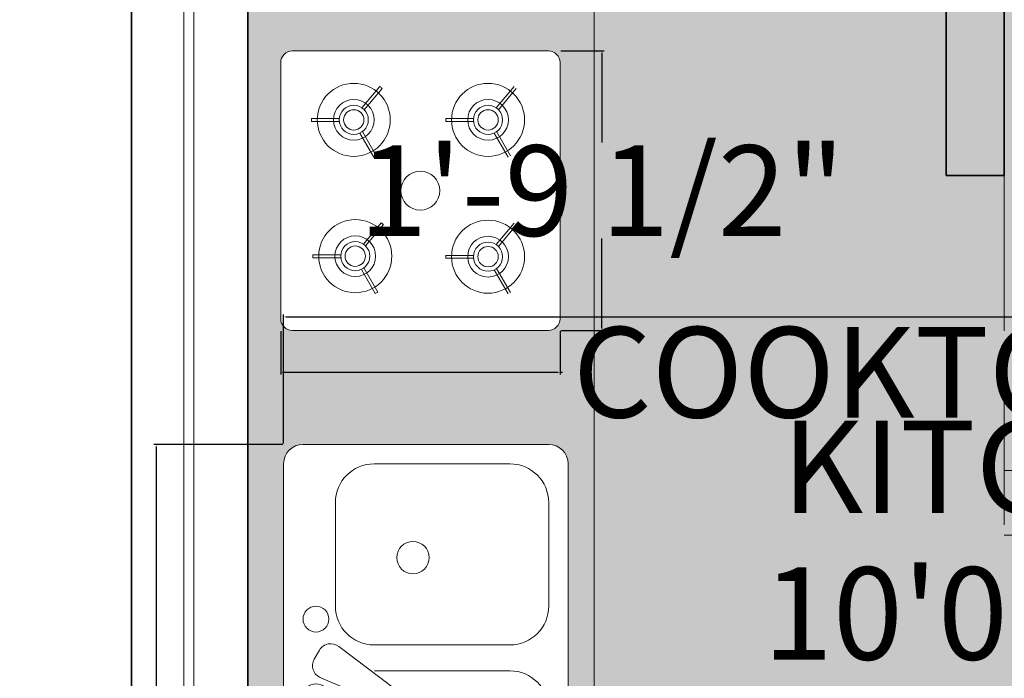
# Model space of a CAD drawing. Units: inches. Extents: x 1316 to 1777, y 813 to 1650.
# Tile 6 of 22: x 1368 to 1445, y 1284 to 1335. Entities that reach past the tile are written whole.
import ezdxf

# ---------------------------------------------------------------- set-up
doc = ezdxf.new("R2010")
doc.units = ezdxf.units.IN
doc.header["$MEASUREMENT"] = 0
doc.linetypes.add('ACAD_ISO02W100', pattern=[15, 12, -3])
for name, color, linetype, lineweight in [('A-ANNO-DIMS', 2, 'Continuous', 18), ('A-AREA-IDEN', 7, 'Continuous', 18), ('A-EQPM', 8, 'Continuous', 18), ('A-FLOR-CASE', 23, 'Continuous', 18), ('A-FLOR-CASE-PATT', 252, 'Continuous', 13), ('A-FLOR-FIXT', 8, 'Continuous', 18), ('A-WALL-OVHD', 250, 'ACAD_ISO02W100', 18), ('A-WALL-PATT', 250, 'Continuous', 13), ('furniture', 23, 'Continuous', 18), ('walls', 250, 'Continuous', 35), ('windows', 141, 'Continuous', 18)]:
    doc.layers.add(name, color=color, linetype=linetype, lineweight=lineweight)
doc.layers.add('A-FLOR-PATT', color=254, linetype='Continuous', lineweight=13, true_color=0xfeeab9)
doc.styles.add('ATT', font='TXT')
doc.styles.get("Standard").update_dxf_attribs({"font": 'arial.ttf'})
doc.dimstyles.get("Standard").update_dxf_attribs({"dimtxt": 7, "dimasz": 0.18, "dimexe": 0.18, "dimexo": 0.0625, "dimgap": 0.09, "dimtad": 0, "dimtih": 1, "dimtoh": 1, "dimzin": 0, "dimdsep": 46, "dimlunit": 3, "dimtxsty": 'Standard', "dimcen": 0.09, "dimadec": 0, "dimazin": 0, "dimtfac": 1, "dimtofl": 0, "dimtmove": 0, "dimatfit": 3, "dimfxl": 1, "dimtolj": 1, "dimtzin": 0, "dimarcsym": 0})

# ---------------------------------------------------------------- blocks, each defined once
blk = doc.blocks.new('15PSNK10')
at = {"color": 0, "linetype": 'ByBlock'}
for p, q in [((20.5, 16.5), (1.5, 16.5)), ((0, 15), (0, -15)), ((7, 15), (17.5, 15)), ((22, -15), (22, 15)), ((4, 4), (4, 12)), ((20.5, 12), (20.5, 4)), ((10.17820310567643, -3.566986483662404), (4.270020000000002, 0.8709410000000019)), ((17.5, 1), (7, 1)), ((2.365550999999996, -0.0988979999999984), (2.768423999999995, 0.5988979999999984)), ((7.038591832997624, -1), (17.5, -1)), ((2.880752999999998, -1.535340000000005), (9.678203105676431, -4.433012483662395)), ((9.678203105676431, -4.433012483662395), (10.17820310567643, -3.566986483662404)), ((4, -12), (4, -4)), ((20.5, -4), (20.5, -12)), ((17.5, -15), (7, -15)), ((1.5, -16.5), (20.5, -16.5))]:
    blk.add_line(p, q, dxfattribs=at)
for centre, radius in [((10, 7.75), 1.25), ((2.5, 3), 1), ((2.5, -3), 1), ((10, -7.75), 1.25)]:
    blk.add_circle(centre, radius, dxfattribs=at)
for centre, radius, start, end in [((1.5, 15), 1.5, 90, 180), ((20.5, 15), 1.5, 0, 90), ((7, 12), 3, 90, 180), ((17.5, 12), 3, 0, 90), ((7, 4), 3, 180, 270), ((17.5, 4), 3, 270, 0), ((3.634449000000003, 0.0988979999999984), 1, 50.537678, 150), ((3.231576000000004, -0.5988979999999984), 1, 150, 249.462322), ((17.5, -4), 3, 0, 90), ((7, -4), 3, 146.6070344853579, 180), ((7, -12), 3, 180, 270), ((17.5, -12), 3, 270, 0), ((1.5, -15), 1.5, 180, 270), ((20.5, -15), 1.5, 270, 0)]:
    blk.add_arc(centre, radius, start, end, dxfattribs=at)
at = {"color": 0, "linetype": 'ByBlock', "style": 'ATT'}
for tag, p, flags in [('ITEM', (0, -26), 3), ('ROOM_NUMBER', (0, -35), 1)]:
    blk.add_attdef(tag, p, '', height=6, dxfattribs=dict(at, flags=flags))
blk = doc.blocks.new('4bstove')
at = {"layer": 'furniture'}
for p, q in [((1452.734651100344, 1446.213675667939), (1452.734651100344, 1448.605619579717)), ((1452.984651100344, 1446.216662390849), (1452.984651100344, 1448.606641539671)), ((1464.44122432111, 1446.341246424268), (1464.44122432111, 1448.733190336046)), ((1464.69122432111, 1446.344233147178), (1464.69122432111, 1448.734212296)), ((1451.73906976938, 1444.448764170567), (1449.669037203066, 1443.253630311174)), ((1451.865811318356, 1444.233263303391), (1449.79463312554, 1443.037468016228)), ((1453.750175383867, 1444.079499707197), (1455.581487244284, 1442.54284660055)), ((1453.910173656299, 1444.271597038143), (1455.741945084313, 1442.734558308493)), ((1463.445642990145, 1444.576334926896), (1461.375610423832, 1443.381201067503)), ((1463.572384539122, 1444.36083405972), (1461.501206346306, 1443.165038772557)), ((1465.456748604633, 1444.207070463526), (1467.288060465049, 1442.670417356879)), ((1465.616746877065, 1444.399167794472), (1467.448518305079, 1442.862129064822)), ((1452.691937061862, 1434.805644860098), (1452.691937061862, 1437.197588771873)), ((1452.941937061862, 1434.808631583008), (1452.941937061862, 1437.19861073183)), ((1464.44122432111, 1434.805644860098), (1464.44122432111, 1437.197588771873)), ((1464.69122432111, 1434.808631583008), (1464.69122432111, 1437.19861073183)), ((1451.696355730898, 1433.040733362724), (1449.626323164584, 1431.845599503333)), ((1463.445642990145, 1433.040733362724), (1461.375610423832, 1431.845599503333)), ((1451.823097279874, 1432.82523249555), (1449.751919087058, 1431.629437208387)), ((1453.707461345386, 1432.671468899352), (1455.538773205802, 1431.134815792708)), ((1453.867459617818, 1432.863566230298), (1455.699231045831, 1431.326527500652)), ((1463.572384539122, 1432.82523249555), (1461.501206346306, 1431.629437208387)), ((1465.456748604633, 1432.671468899352), (1467.288060465049, 1431.134815792708)), ((1465.616746877065, 1432.863566230298), (1467.448518305079, 1431.326527500652))]:
    blk.add_line(p, q, dxfattribs=at)
for points in [[(1447.502363082413, 1427.379846129004), (1469.502363082413, 1427.379846129004, 0.4142135623730951), (1470.502363082413, 1428.379846129004), (1470.502363082413, 1450.379846129006, 0.4142135623730951), (1469.502363082413, 1451.379846129006), (1447.502363082413, 1451.379846129006, 0.4142135623730966), (1446.502363082413, 1450.379846129006), (1446.502363082413, 1428.379846129004, 0.4142135623730935)], [(1453.749508788236, 1444.971524377983, 1), (1451.999508788236, 1444.971524377983, 1)], [(1465.456082009002, 1445.099095134312, 1), (1463.706082009001, 1445.099095134312, 1)], [(1453.706794749754, 1433.563493570142, 1), (1451.956794749754, 1433.563493570142, 1)], [(1465.456082009002, 1433.563493570142, 1), (1463.706082009001, 1433.563493570142, 1)]]:
    blk.add_lwpolyline(points, format="xyb", close=True, dxfattribs=at)
for points in [[(1454.124508788236, 1444.971524377983, 0.9999999673531919), (1451.624508788236, 1444.971524377983, 0.9999999673531919), (1454.124508788236, 1444.971524377983, 0.9999999673531919)], [(1465.831082009002, 1445.099095134312, 1), (1463.331082009001, 1445.099095134312, 1), (1465.831082009002, 1445.099095134312, 1)], [(1454.081794749754, 1433.563493570142, 0.9999999673531919), (1451.581794749754, 1433.563493570142, 0.9999999673531919), (1454.081794749754, 1433.563493570142, 0.9999999673531919)], [(1465.831082009002, 1433.563493570142, 1), (1463.331082009001, 1433.563493570142, 1), (1465.831082009002, 1433.563493570142, 1)]]:
    blk.add_lwpolyline(points, format="xyb", dxfattribs=at)
for centre, radius in [((1452.874508788236, 1444.971524377983), 3.136785408586831), ((1464.581082009001, 1445.099095134312), 3.136785408586831), ((1452.874508788236, 1444.971524377983), 1.75), ((1464.581082009001, 1445.099095134312), 1.75), ((1458.502363082413, 1439.379846129004), 1.670451188942094), ((1452.831794749754, 1433.563493570142), 3.136785408586831), ((1464.581082009001, 1433.563493570142), 3.136785408586831), ((1452.831794749754, 1433.563493570142), 1.75), ((1464.581082009001, 1433.563493570142), 1.75)]:
    blk.add_circle(centre, radius, dxfattribs=at)
for centre, start, end in [((1452.874508788236, 1444.971524377983), 88.2644962424337, 92.20393308675509), ((1464.581082009001, 1445.099095134312), 88.2644962424337, 92.20393308675509), ((1452.874508788236, 1444.971524377983), 208.1879938332412, 212.1274126783975), ((1464.581082009001, 1445.099095134312), 208.1879938332412, 212.1274126783975), ((1452.874508788236, 1444.971524377983), 318.1018185131579, 322.0412255005968), ((1464.581082009001, 1445.099095134312), 318.1018185131579, 322.0412255005968), ((1452.831794749754, 1433.563493570142), 88.2644962424337, 92.20393308675509), ((1464.581082009001, 1433.563493570142), 88.2644962424337, 92.20393308675509)]:
    blk.add_arc(centre, 3.636785408586831, start, end, dxfattribs=at)
blk = doc.blocks.new('stove')
at = {"layer": 'furniture', "xscale": 0.9, "yscale": 0.9, "zscale": 0.9, "rotation": 89.99999999999999}
blk.add_blockref('4bstove', (1295.441862106323, -1312.652126789093), dxfattribs=at)
blk = doc.blocks.new('*D36')
at = {"layer": 'A-ANNO-DIMS', "color": 0, "lineweight": -2, "transparency": 16777216}
for p, q in [((1416.108011424953, 1349.392697936214), (1416.108011424953, 1345.951925450247)), ((1438.2631613314, 1349.392697936214), (1438.2631613314, 1345.951925450247)), ((1416.288011424953, 1346.131925450247), (1438.0831613314, 1346.131925450247)), ((1438.2631613314, 1346.131925450247), (1438.443161331401, 1346.131925450247))]:
    blk.add_line(p, q, dxfattribs=at)
at = {"layer": 'A-ANNO-DIMS', "color": 0, "transparency": 16777216}
for points in [[(1416.288011424953, 1346.161925450247), (1416.288011424953, 1346.101925450247), (1416.108011424953, 1346.131925450247)], [(1438.0831613314, 1346.161925450247), (1438.0831613314, 1346.101925450247), (1438.2631613314, 1346.131925450247)]]:
    blk.add_solid(points, dxfattribs=at)
at = {"layer": 'Defpoints', "color": 0, "transparency": 16777216}
for p in [(1416.108011424953, 1349.455197936214), (1438.2631613314, 1349.455197936214), (1438.2631613314, 1346.131925450247)]:
    blk.add_point(p, dxfattribs=at)
at = {"layer": 'A-ANNO-DIMS', "color": 0, "transparency": 16777216, "insert": (1493.434934864825, 1346.131925450247), "char_height": 7, "attachment_point": 5}
blk.add_mtext('\\A1;WALL BASIN 1\'-10" TYP.', dxfattribs=at)
blk = doc.blocks.new('*D40')
at = {"layer": 'A-ANNO-DIMS', "color": 0, "lineweight": -2, "transparency": 16777216}
for p, q in [((1388.838253781963, 1302.162642632137), (1388.838253781963, 1312.140959778822)), ((1389.018253781963, 1311.960959778821), (1454.39703475986, 1311.960959778821)), ((1454.57703475986, 1302.162642632137), (1454.57703475986, 1312.140959778822)), ((1454.57703475986, 1311.960959778821), (1454.757034759859, 1311.960959778821))]:
    blk.add_line(p, q, dxfattribs=at)
at = {"layer": 'A-ANNO-DIMS', "color": 0, "transparency": 16777216}
for points in [[(1389.018253781963, 1311.990959778821), (1389.018253781963, 1311.930959778822), (1388.838253781963, 1311.960959778821)], [(1454.39703475986, 1311.990959778821), (1454.39703475986, 1311.930959778822), (1454.57703475986, 1311.960959778821)]]:
    blk.add_solid(points, dxfattribs=at)
at = {"layer": 'Defpoints', "color": 0, "transparency": 16777216}
for p in [(1454.57703475986, 1311.960959778821), (1388.838253781963, 1302.100142632137), (1454.57703475986, 1302.100142632137)]:
    blk.add_point(p, dxfattribs=at)
at = {"layer": 'A-ANNO-DIMS', "color": 0, "transparency": 16777216, "insert": (1507.740963818523, 1311.960959778821), "char_height": 7, "attachment_point": 5}
blk.add_mtext('\\A1;KITCHEN SINK 5\'-5 1/2"', dxfattribs=at)
blk = doc.blocks.new('*D41')
at = {"layer": 'A-ANNO-DIMS', "color": 0, "lineweight": -2, "transparency": 16777216}
for p, q in [((1388.775753781963, 1302.100142632137), (1378.797436635279, 1302.100142632137)), ((1378.977436635279, 1301.920142632137), (1378.977436635279, 1279.143834211486)), ((1378.977436635279, 1249.068153348815), (1378.977436635279, 1271.844461769467)), ((1388.775753781963, 1248.888153348815), (1378.797436635279, 1248.888153348815))]:
    blk.add_line(p, q, dxfattribs=at)
at = {"layer": 'A-ANNO-DIMS', "color": 0, "transparency": 16777216}
for points in [[(1378.947436635279, 1301.920142632137), (1379.007436635279, 1301.920142632137), (1378.977436635279, 1302.100142632137)], [(1378.947436635279, 1249.068153348815), (1379.007436635279, 1249.068153348815), (1378.977436635279, 1248.888153348815)]]:
    blk.add_solid(points, dxfattribs=at)
at = {"layer": 'Defpoints', "color": 0, "transparency": 16777216}
for p in [(1378.977436635279, 1302.100142632137), (1388.838253781963, 1302.100142632137), (1388.838253781963, 1248.888153348815)]:
    blk.add_point(p, dxfattribs=at)
at = {"layer": 'A-ANNO-DIMS', "color": 0, "transparency": 16777216, "insert": (1378.977436635279, 1275.494147990476), "char_height": 7, "attachment_point": 5}
blk.add_mtext('\\A1;4\'-5"', dxfattribs=at)
blk = doc.blocks.new('*D42')
at = {"layer": 'A-ANNO-DIMS', "color": 0, "lineweight": -2, "transparency": 16777216}
for p, q in [((1388.610422891291, 1310.852265372921), (1388.610422891291, 1307.49476537292)), ((1410.210422891293, 1310.852265372921), (1410.210422891293, 1307.49476537292)), ((1388.790422891291, 1307.674765372921), (1410.030422891293, 1307.674765372921)), ((1410.210422891293, 1307.674765372921), (1410.390422891293, 1307.674765372921))]:
    blk.add_line(p, q, dxfattribs=at)
at = {"layer": 'A-ANNO-DIMS', "color": 0, "transparency": 16777216}
for points in [[(1388.790422891291, 1307.704765372921), (1388.790422891291, 1307.644765372921), (1388.610422891291, 1307.674765372921)], [(1410.030422891293, 1307.704765372921), (1410.030422891293, 1307.644765372921), (1410.210422891293, 1307.674765372921)]]:
    blk.add_solid(points, dxfattribs=at)
at = {"layer": 'Defpoints', "color": 0, "transparency": 16777216}
for p in [(1388.610422891291, 1310.914765372921), (1410.210422891293, 1310.914765372921), (1410.210422891293, 1307.674765372921)]:
    blk.add_point(p, dxfattribs=at)
at = {"layer": 'A-ANNO-DIMS', "color": 0, "transparency": 16777216, "insert": (1453.707571595249, 1307.674765372921), "char_height": 7, "attachment_point": 5}
blk.add_mtext('\\A1;COOKTOP 1\'-9 1/2"', dxfattribs=at)
blk = doc.blocks.new('*D43')
at = {"layer": 'A-ANNO-DIMS', "color": 0, "lineweight": -2, "transparency": 16777216}
for p, q in [((1410.272922891293, 1332.514765372921), (1413.630422891294, 1332.514765372921)), ((1413.450422891294, 1332.334765372921), (1413.450422891294, 1325.42413781494)), ((1413.450422891294, 1311.094765372921), (1413.450422891294, 1318.005392930902)), ((1410.272922891293, 1310.914765372921), (1413.630422891294, 1310.914765372921))]:
    blk.add_line(p, q, dxfattribs=at)
at = {"layer": 'A-ANNO-DIMS', "color": 0, "transparency": 16777216}
for points in [[(1413.420422891294, 1332.334765372921), (1413.480422891294, 1332.334765372921), (1413.450422891294, 1332.514765372921)], [(1413.420422891294, 1311.094765372921), (1413.480422891294, 1311.094765372921), (1413.450422891294, 1310.914765372921)]]:
    blk.add_solid(points, dxfattribs=at)
at = {"layer": 'Defpoints', "color": 0, "transparency": 16777216}
for p in [(1410.210422891293, 1332.514765372921), (1413.450422891294, 1332.514765372921), (1410.210422891293, 1310.914765372921)]:
    blk.add_point(p, dxfattribs=at)
at = {"layer": 'A-ANNO-DIMS', "color": 0, "transparency": 16777216, "insert": (1413.450422891294, 1321.714765372921), "char_height": 7, "attachment_point": 5}
blk.add_mtext('\\A1;1\'-9 1/2"', dxfattribs=at)

msp = doc.modelspace()

# ---------------------------------------------------------------- hatches: boundary and pattern name
at = {"layer": 'A-FLOR-CASE-PATT'}
h = msp.add_hatch(color=256, dxfattribs=at)
h.dxf.hatch_style = 1
h.paths.add_polyline_path([(1412.858226839809, 1346.928610372446), (1440.064450217018, 1346.928610372446), (1440.064450217018, 1365.369300926962), (1438.2631613314, 1365.369300926962), (1438.2631613314, 1349.455197936214), (1416.108011424953, 1349.455197936214), (1416.108011424953, 1365.369300926962), (1386.064450217018, 1365.369300926962), (1386.064450217018, 1245.369300926962), (1412.858226839809, 1245.369300926962)])
h.paths.add_polyline_path([(1409.310422891292, 1332.514765372921, -0.4142135623730951), (1410.210422891292, 1331.614765372921), (1410.210422891292, 1311.814765372921, -0.414213562373094), (1409.310422891292, 1310.914765372921), (1389.51042289129, 1310.914765372921, -0.4142135623730959), (1388.61042289129, 1311.814765372921), (1388.61042289129, 1331.614765372921, -0.4142135623730951), (1389.51042289129, 1332.514765372921)], flags=16)
h.paths.add_polyline_path([(1395.986900854525, 1329.42133126595), (1396.276368249055, 1329.76630507332, -0.0171905986958355), (1396.448908786205, 1329.621893017294), (1396.159470211814, 1329.276953556429, -0.2116405901053515), (1397.086205654243, 1327.18561240685, -0.2564460938474173), (1395.778569555149, 1324.8037474367), (1396.003749512095, 1324.413724310425, -0.0171906504505625), (1395.809203446643, 1324.300687980197), (1395.584072921188, 1324.69062548862, -0.550570801787435), (1391.442799396982, 1327.059740487748), (1390.992413104956, 1327.059740487748, -0.0171907290098312), (1390.991493340996, 1327.284740487748), (1391.441732803486, 1327.284740487748, -0.6105283005508269)], flags=0)
h.paths.add_polyline_path([(1395.838098786515, 1327.18561240685, -1), (1392.688098786514, 1327.18561240685, -1)], flags=0)
h.paths.add_polyline_path([(1394.263098786514, 1328.310612406851, -1), (1394.263098786514, 1326.06061240685, -1)], flags=0)
h.paths.add_polyline_path([(1394.263098786514, 1327.973112406851, -1), (1394.263098786514, 1326.39811240685, -1)], flags=0)
h.paths.add_polyline_path([(1407.468247061996, 1327.18561240685, -0.9779444631718501), (1401.824840804736, 1327.059740487748), (1401.37445451271, 1327.059740487748, -0.0171907290098312), (1401.373534748749, 1327.284740487748), (1401.823774211239, 1327.284740487748, -0.9825922263687022)], flags=0)
h.paths.add_polyline_path([(1406.220140194268, 1327.18561240685, -1), (1403.070140194268, 1327.18561240685, -1)], flags=0)
h.paths.add_polyline_path([(1404.645140194268, 1328.310612406851, -1), (1404.645140194268, 1326.06061240685, -1)], flags=0)
h.paths.add_polyline_path([(1404.645140194268, 1327.973112406851, -1), (1404.645140194268, 1326.39811240685, -1)], flags=0)
h.paths.add_polyline_path([(1400.91382896134, 1321.714765372921, -1), (1397.907016821244, 1321.714765372921, -1)], flags=0)
h.paths.add_polyline_path([(1396.101714535222, 1318.885415367262), (1396.391181929752, 1319.230389174631, -0.0171905986957908), (1396.563722466901, 1319.085977118605), (1396.274283892511, 1318.74103765774, -0.2116405901053402), (1397.201019334939, 1316.649696508162, -0.2564460938474829), (1395.893383235845, 1314.267831538011), (1396.11856319279, 1313.877808411735, -0.0171906504505387), (1395.924017127339, 1313.764772081509), (1395.698886601884, 1314.154709589932, -0.5505708017872751), (1391.557613077679, 1316.523824589059), (1391.107226785653, 1316.523824589059, -0.0171907290098486), (1391.106307021692, 1316.748824589059), (1391.556546484182, 1316.748824589059, -0.6105283005510082)], flags=0)
h.paths.add_polyline_path([(1395.952912467211, 1316.649696508162, -1), (1392.802912467211, 1316.649696508162, -1)], flags=0)
h.paths.add_polyline_path([(1407.468247061996, 1316.611253873528, -0.9779444631716472), (1401.824840804736, 1316.485381954425), (1401.37445451271, 1316.485381954425, -0.0171907290098486), (1401.373534748749, 1316.710381954425), (1401.823774211239, 1316.710381954425, -0.9825922263688615)], flags=0)
h.paths.add_polyline_path([(1394.377912467211, 1317.774696508162, -0.9999999703822144), (1394.377912467211, 1315.524696508162, -0.9999999703822144)], flags=0)
h.paths.add_polyline_path([(1394.377912467211, 1317.437196508162, -1), (1394.377912467211, 1315.862196508162, -1)], flags=0)
h.paths.add_polyline_path([(1406.220140194268, 1316.611253873528, -1), (1403.070140194268, 1316.611253873528, -1)], flags=0)
h.paths.add_polyline_path([(1404.645140194268, 1315.486253873528, -0.9999999703822144), (1404.645140194268, 1317.736253873528, -0.9999999703822144)], flags=0)
h.paths.add_polyline_path([(1404.645140194268, 1317.398753873528, -1), (1404.645140194268, 1315.823753873528, -1)], flags=0)
h.paths.add_polyline_path([(1409.338253781963, 1302.100142632137, -0.4142135623730951), (1410.838253781963, 1300.600142632137), (1410.838253781963, 1270.600142632137, -0.4142135623730951), (1409.338253781963, 1269.100142632137), (1390.338253781963, 1269.100142632137, -0.4142135623730951), (1388.838253781963, 1270.600142632137), (1388.838253781963, 1300.600142632137, -0.4142135623730951), (1390.338253781963, 1302.100142632137)], flags=16)
h.paths.add_polyline_path([(1395.838253781963, 1300.600142632137), (1406.338253781963, 1300.600142632137, -0.4142135623730951), (1409.338253781963, 1297.600142632137), (1409.338253781963, 1289.600142632137, -0.4142135623730951), (1406.338253781963, 1286.600142632137), (1395.838253781963, 1286.600142632137, -0.4142135623730951), (1392.838253781963, 1289.600142632137), (1392.838253781963, 1297.600142632137, -0.4142135623730951)], flags=0)
h.paths.add_polyline_path([(1400.088253781963, 1293.350142632137, -1), (1397.588253781963, 1293.350142632137, -1)], flags=0)
h.paths.add_polyline_path([(1392.338253781963, 1288.600142632137, -1), (1390.338253781963, 1288.600142632137, -1)], flags=0)
h.paths.add_polyline_path([(1393.037126479862, 1286.524525876857), (1399.01645688764, 1282.033156148475), (1398.51645688764, 1281.167130148475), (1391.719002681245, 1284.064804380225, -0.4631994748411593), (1391.203386694108, 1285.500520483254), (1391.606259694108, 1286.198316483253, -0.4369421512224802)], flags=0)
h.paths.add_polyline_path([(1392.338253781963, 1282.600142632137, -1), (1390.338253781963, 1282.600142632137, -1)], flags=0)
h.paths.add_polyline_path([(1400.088253781963, 1277.850142632137, -1), (1397.588253781963, 1277.850142632137, -1)], flags=0)
at = {"layer": 'A-FLOR-PATT'}
h = msp.add_hatch(color=256, dxfattribs=at)
h.dxf.hatch_style = 1
h.paths.add_polyline_path([(1567.673142217696, 1281.369300926962), (1651.673142217696, 1281.369300926962), (1651.673142217696, 1365.369300926962), (1597.673142217696, 1365.369300926962), (1597.673142217696, 1429.869300926962), (1570.345136951899, 1429.869300926962), (1570.345136951899, 1471.869300926962), (1510.345136951899, 1471.869300926962), (1510.345136951899, 1429.869300926962), (1444.564450217018, 1429.869300926962), (1444.564450217018, 1322.882360660317), (1444.564450217018, 1300.087519887597), (1510.564450217018, 1300.087519887597), (1510.564450217018, 1295.093869264817), (1510.564450217018, 1240.869300926962), (1386.064450217018, 1240.869300926962), (1386.064450217018, 1171.184826128129), (1400.961298831769, 1171.184826128129), (1400.961298831769, 1106.74181853581), (1386.064450217018, 1106.74181853581), (1386.064450217018, 1072.869300926962), (1510.564450217018, 1072.869300926962), (1510.564450217018, 1040.172951843256), (1541.068383692007, 1040.172951843256, -0.367085007058701), (1572.764174999282, 1069.546549507821), (1572.764174999282, 1069.578525976929), (1574.225256623933, 1069.578525976929), (1574.225256623933, 1040.172951843256), (1616.037285953149, 1040.172951843256), (1616.037285953149, 1086.627161740109), (1616.037285953149, 1103.704513499145), (1613.066060418845, 1105.234780569291), (1616.037285953149, 1106.685539866415), (1616.037285953149, 1123.869300926962), (1567.673142217696, 1123.869300926962)])
h.paths.add_polyline_path([(1508.987494855724, 1198.018101264616), (1511.117481528599, 1198.018101264616), (1511.117481528599, 1200.148087937491), (1532.594847146751, 1200.148087937491), (1532.594847146751, 1198.018101264616), (1534.724833819626, 1198.018101264616), (1534.724833819626, 1176.008238978245), (1530.464860473877, 1176.008238978245), (1530.464860473877, 1176.71823453587), (1513.247468201473, 1176.71823453587), (1513.247468201473, 1176.008238978245), (1508.987494855724, 1176.008238978245)], flags=16)
h.paths.add_polyline_path([(1505.978911344017, 1151.314990471522), (1521.503967005494, 1151.314990471522), (1521.503967005494, 1123.622553675171), (1505.978911344017, 1123.622553675171)], flags=16)
h.paths.add_polyline_path([(1507.734238645614, 1150.100746953806, -1), (1506.932299902515, 1150.100746953806, -1)], flags=0)
h.paths.add_polyline_path([(1512.288074001727, 1138.353334368216), (1512.279600715468, 1138.392440283947), (1512.219350358134, 1138.376242249414)], flags=0)
h.paths.add_polyline_path([(1511.538708600003, 1138.926307509397), (1511.801586230713, 1138.967144364025), (1511.816822451641, 1139.269704188439), (1511.606794574277, 1139.246286533845)], flags=0)
h.paths.add_polyline_path([(1513.744555260512, 1140.234298321423), (1513.680232363733, 1139.885116881769), (1514.013725426534, 1140.045442118172), (1513.85452204526, 1140.307851476896)], flags=0)
h.paths.add_polyline_path([(1513.759454991183, 1139.088508933479), (1514.004707571892, 1139.255238426424), (1513.806733823314, 1139.482778214552), (1513.564128907831, 1139.327271464974)], flags=0)
h.paths.add_polyline_path([(1514.219475210051, 1138.385213274156), (1514.335730050378, 1138.330012877603), (1514.544443105969, 1138.319719602207), (1514.802071501717, 1138.873746829037), (1514.451386945615, 1138.715560522777)], flags=0)
h.paths.add_polyline_path([(1514.576784523415, 1137.439218133731), (1514.572807725035, 1137.400121795131), (1514.699202201671, 1137.400121795131), (1514.696265725507, 1137.401958254237)], flags=0)
h.paths.add_polyline_path([(1512.259630054145, 1136.199252443718), (1512.198645006043, 1136.399020086717), (1512.031969302785, 1136.324884611944), (1512.095408670439, 1136.101205019573), (1512.257489338984, 1136.192116726515)], flags=0)
h.paths.add_polyline_path([(1512.643663084783, 1137.273739653883), (1512.355504649132, 1137.230281342332), (1512.431954114942, 1137.048783229095), (1512.702875297586, 1137.092989450977)], flags=0)
h.paths.add_polyline_path([(1513.048588650928, 1137.592520798729), (1512.979298324136, 1137.799799709794), (1512.842806872769, 1137.757466697763), (1512.887278702865, 1137.556025839099)], flags=0)
h.paths.add_polyline_path([(1513.269281623239, 1138.555876366321), (1513.570749546786, 1137.962332598873), (1513.458764523686, 1136.814048268166), (1513.212081965274, 1137.877990637943), (1513.032322366809, 1138.442602014432)], flags=0)
h.paths.add_polyline_path([(1514.891020715756, 1136.377090047208), (1514.695899864911, 1136.400535518201), (1514.682939550409, 1136.245500587688), (1514.870369662043, 1136.165423867704)], flags=0)
h.paths.add_polyline_path([(1514.142311807212, 1137.292647657223), (1514.047049214511, 1136.74320071616), (1514.270411313405, 1136.750949401328), (1514.327746372416, 1137.265481105849)], flags=0)
h.paths.add_polyline_path([(1515.361925908058, 1138.975942407129), (1515.333738674027, 1138.638448296537), (1515.595602136156, 1138.588081597507), (1515.627104749056, 1138.931608018565)], flags=0)
h.paths.add_polyline_path([(1537.284795120854, 1177.912388692567), (1537.994790678479, 1177.912388692567), (1537.994790678479, 1195.129780964971), (1537.284795120854, 1195.129780964971), (1537.284795120854, 1199.38975431072), (1559.294657407225, 1199.38975431072), (1559.294657407225, 1197.259767637845), (1561.4246440801, 1197.259767637845), (1561.4246440801, 1175.782402019693), (1559.294657407225, 1175.782402019693), (1559.294657407225, 1173.652415346818), (1559.378615070445, 1173.652415346818), (1559.378615070445, 1171.514303738793), (1561.51672667847, 1171.514303738793), (1561.51672667847, 1098.818509065945), (1559.378615070445, 1098.818509065945), (1559.378615070445, 1096.68039745792), (1537.284795120854, 1096.68039745792), (1537.284795120854, 1100.95662067397), (1537.997498990196, 1100.95662067397), (1537.997498990196, 1169.376192130768), (1537.284795120854, 1169.376192130768), (1537.284795120854, 1173.652415346818)], flags=16)
h.paths.add_polyline_path([(1518.623279367581, 1345.565265318288), (1519.133216999197, 1345.479657117201), (1519.133247129367, 1345.484585273925), (1518.623292796693, 1345.567461813277)], flags=16)
h.paths.add_polyline_path([(1518.798043157878, 1374.150014517315), (1519.307980789494, 1374.064406316228), (1519.308010919664, 1374.069334472953), (1518.79805658699, 1374.152211012305)], flags=16)
h.paths.add_polyline_path([(1537.763945546351, 1413.501272593833), (1537.678419015976, 1412.991334462891), (1537.683273643974, 1412.991304782267), (1537.76615767817, 1413.501259069119)], flags=16)
h.paths.add_polyline_path([(1572.904903294898, 1373.821409718101), (1573.926762419731, 1373.974678074354), (1574.026627442758, 1390.308820473798), (1573.007147246318, 1390.474521481455), (1573.006718884663, 1390.474591095266)], flags=16)
h.paths.add_polyline_path([(1572.730139504601, 1345.236660519073), (1573.751998629434, 1345.389928875326), (1573.851863652461, 1361.72407127477), (1572.832383456021, 1361.889772282427), (1572.831955094366, 1361.889841896238)], flags=16)
h.paths.add_polyline_path([(1537.210658487583, 1322.64259197221), (1537.363943428096, 1321.620732745983), (1553.69808582754, 1321.520867722956), (1553.863838585734, 1322.540776390265)], flags=16)
h.paths.add_polyline_path([(1535.907853535946, 1331.328394679552), (1527.214399285865, 1331.381545435045), (1527.663791889487, 1404.885186232545), (1564.415612288236, 1404.660489930734), (1563.966219684615, 1331.156849133235), (1555.272745017813, 1331.210000013553), (1553.946716560728, 1323.050730714162), (1537.134020158137, 1323.153521560007)], flags=16)
h.paths.add_polyline_path([(1536.149948378398, 1336.502989385165), (1536.235164066325, 1337.571577967879), (1536.323287084786, 1338.628101895201), (1536.410786509507, 1339.662781903015), (1536.494625364907, 1340.6698173033), (1536.573878305868, 1341.65983134291), (1536.648126641431, 1342.647834135966), (1536.716972722469, 1343.648937760143), (1536.780017027388, 1344.677948027938), (1536.836830656389, 1345.749875115879), (1536.91349345135, 1347.47536960008), (1536.930181129876, 1348.082213381731), (1536.86671979596, 1346.313806322279), (1536.754065794645, 1344.188314997416), (1536.618602559507, 1342.21851898877), (1536.494625364906, 1340.669817303289), (1536.410786509508, 1339.662781903024), (1536.323287084785, 1338.628101895196), (1536.235164066325, 1337.571577967878), (1536.149948378398, 1336.502989385167), (1536.071202820108, 1335.432319400725), (1536.002480605875, 1334.369653419014), (1535.917201218224, 1332.754159960459), (1535.909282823342, 1332.307756473361), (1535.96435308899, 1333.780079645636), (1536.071202820108, 1335.432319400726)], flags=0)
h.paths.add_polyline_path([(1540.411728678358, 1338.345220732376), (1540.538507986221, 1339.036732867615), (1540.667450686668, 1339.758144792479), (1540.798139602249, 1340.51803480286), (1540.930104638842, 1341.324675241543), (1541.06290820131, 1342.186644529235), (1541.195663950278, 1343.109256879628), (1541.325751198274, 1344.084667215432), (1541.450112594895, 1345.102072455087), (1541.565699126105, 1346.150363189455), (1541.669432399664, 1347.218634373414), (1541.758274858692, 1348.295980712192), (1541.829158319786, 1349.371497098253), (1541.87902418423, 1350.434176273261), (1541.905658245644, 1351.475864398132), (1541.910264078201, 1352.499718972741), (1541.894848813054, 1353.511751165878), (1541.861450207875, 1354.517971959091), (1541.812104772023, 1355.524188157142), (1541.748831093802, 1356.536615043187), (1541.673675267255, 1357.560957271187), (1541.551221046702, 1359.062282646612), (1541.495486505545, 1359.670454934914), (1541.588655256529, 1358.603328035907), (1541.721318618915, 1356.976835527602), (1541.846114060333, 1354.980013725856), (1541.912433480836, 1352.981966815021), (1541.903299375855, 1350.951498912638), (1541.805645357175, 1348.870418133965), (1541.627733180341, 1346.712969607265), (1541.39605931794, 1344.611846225434), (1541.135168242209, 1342.655652549989), (1540.871929016276, 1340.947082961546), (1540.617179283622, 1339.465841984599), (1540.411728678363, 1338.345220732389), (1540.287580984743, 1337.67502977883), (1540.166494164132, 1337.01788791383), (1540.048925605183, 1336.365114503449), (1539.936674201221, 1335.710368832696), (1539.836864251217, 1335.055036635329), (1539.758020939376, 1334.402536924379), (1539.708629238703, 1333.756391050932), (1539.697173498044, 1333.120018277682), (1539.75093556766, 1332.162191347439), (1539.822087714565, 1331.89006440645), (1539.690956844971, 1332.774679737417), (1539.713650637448, 1334.035332547662), (1539.86680860596, 1335.30285325234), (1540.085210789094, 1336.576760560778), (1540.287580984743, 1337.67502977883)], flags=0)
h.paths.add_polyline_path([(1545.598581542273, 1331.583674047033), (1545.601408931398, 1331.616855477121), (1545.614142276281, 1331.689058908809), (1545.736718477884, 1332.197227143153), (1545.766951209007, 1332.331509735297), (1545.840044120643, 1332.681341212682), (1545.924609388668, 1333.114205605127), (1546.015565858785, 1333.613901317454), (1546.107830504227, 1334.163920489319), (1546.196310713542, 1334.747857411176), (1546.27592408412, 1335.349306311069), (1546.341588213349, 1335.951861417042), (1546.388220074462, 1336.539014868746), (1546.411904372759, 1337.098233262493), (1546.413511757999, 1337.631655211558), (1546.395048737181, 1338.145189796344), (1546.358553067975, 1338.644847998394), (1546.30606313221, 1339.136742887642), (1546.239595021565, 1339.626681393686), (1546.161196702551, 1340.120674435653), (1546.072884891005, 1340.624631031533), (1545.887738197254, 1341.63015699768), (1545.717659533451, 1342.62070013092), (1545.546853733249, 1343.94500888803), (1545.431881256549, 1345.533720124316), (1545.403899849759, 1347.401905451854), (1545.417510423816, 1348.013069267128), (1545.410556413592, 1346.957478372932), (1545.425070640934, 1345.988432507364), (1545.462877367243, 1345.105410056077), (1545.521092971858, 1344.300975918152), (1545.595702123642, 1343.566272620922), (1545.68263719895, 1342.892238827028), (1545.777872657803, 1342.270017126221), (1545.877351709551, 1341.690648207114), (1545.977037981224, 1341.145172633476), (1546.133225269608, 1340.296924301995), (1546.32712189736, 1339.07516870602), (1546.43378476773, 1337.614859053002), (1546.377188266119, 1336.278538916938), (1546.246417261819, 1335.078542247844), (1546.032296532176, 1333.665423983985), (1545.840044120643, 1332.681341212682), (1545.766951209007, 1332.331509735297)], flags=0)
h.paths.add_polyline_path([(1551.802739251137, 1337.655775652498), (1551.96257269545, 1338.249893918501), (1552.102195298518, 1338.801154932478), (1552.224958021371, 1339.338328209144), (1552.330696453755, 1339.864579612065), (1552.418402861907, 1340.377056720641), (1552.487067639598, 1340.872600849098), (1552.535672844225, 1341.34835963925), (1552.563199284875, 1341.801276556129), (1552.568639227787, 1342.228499179132), (1552.550972857889, 1342.626868884903), (1552.509678498417, 1342.994551203202), (1552.446288501197, 1343.33337442512), (1552.362792521005, 1343.646491244529), (1552.261208966661, 1343.936747902882), (1552.143557495304, 1344.207194818415), (1552.011836098078, 1344.460678357413), (1551.868075265113, 1344.700350964085), (1551.746105860759, 1344.881722683215), (1550.887297650741, 1346.05192221882), (1550.42788872704, 1347.125680184261), (1550.183287427721, 1348.353333686171), (1550.047936052465, 1349.632359022536), (1549.978096005541, 1351.223542107026), (1549.974102148838, 1353.140827975589), (1549.989226669163, 1353.748427546368), (1549.975058438592, 1352.681752708607), (1549.977087298692, 1351.70778065901), (1549.995607655661, 1350.824569845699), (1550.030618304039, 1350.026913573531), (1550.082058657804, 1349.309911787039), (1550.149928759809, 1348.668561967865), (1550.234168024029, 1348.097964060535), (1550.334775869163, 1347.593013458303), (1550.451691709185, 1347.148810105696), (1550.584412233058, 1346.759844100773), (1550.73038050297, 1346.418678345312), (1550.88655602074, 1346.117266144286), (1551.049909745336, 1345.847764917032), (1551.217401178577, 1345.602127968521), (1551.385990446439, 1345.372410692116), (1551.55262809021, 1345.150770631988), (1552.000038284146, 1344.537104232464), (1552.453505275841, 1343.494713960715), (1552.591463897673, 1342.266339273388), (1552.508711326437, 1340.904737898757), (1552.245597777252, 1339.367339734202), (1551.924893638995, 1338.101128644033), (1551.618511514029, 1336.984114361546), (1551.405674157756, 1336.200020283199), (1551.009764092749, 1334.698598399404), (1550.877399289293, 1334.154667887629), (1551.263664389663, 1335.676855458292), (1551.618511514027, 1336.984114361536)], flags=0)
h.paths.add_polyline_path([(1558.642358998526, 1348.348341932098), (1558.795153425402, 1348.811416841303), (1558.918173552255, 1349.215358215379), (1559.008026171039, 1349.574581801048), (1559.061298904339, 1349.903707646641), (1559.075825921932, 1350.214183320864), (1559.054343192669, 1350.505992096326), (1559.00083323259, 1350.775944766007), (1558.919250427844, 1351.021260663692), (1558.81356708563, 1351.238750644777), (1558.687756761463, 1351.425429741436), (1558.545793010855, 1351.578312985846), (1558.391628971643, 1351.694415535011), (1558.228764001313, 1351.771674150153), (1558.05869086465, 1351.812121548804), (1557.882428128411, 1351.81871217754), (1557.700994359352, 1351.79440048294), (1557.515397915392, 1351.742140973996), (1557.326668820441, 1351.665092211649), (1557.135793766425, 1351.566004652943), (1556.943823194933, 1351.44803673399), (1556.751584825563, 1351.314654529213), (1556.741969848742, 1351.307485185875), (1556.174649390243, 1350.878470713214), (1555.982386678774, 1350.741107061228), (1555.790208852573, 1350.61762743028), (1555.103431920574, 1350.247624890473), (1554.019478994433, 1350.696346369238), (1553.658410413117, 1351.73359972735), (1553.592207666961, 1352.861368347784), (1553.704659497418, 1354.248209262139), (1553.753119918252, 1354.656598557367), (1553.684819216316, 1354.00352392911), (1553.637913725648, 1353.425049987856), (1553.614699631385, 1352.917691559993), (1553.614827379228, 1352.476039895736), (1553.637249468889, 1352.094077959223), (1553.680938817757, 1351.765788589762), (1553.744858758541, 1351.485256777466), (1553.82798220863, 1351.246465361642), (1553.929261667735, 1351.043397306428), (1554.04767130156, 1350.870239627912), (1554.182026927633, 1350.721997047951), (1554.330490954936, 1350.598680801359), (1554.491077653114, 1350.501119766308), (1554.661792955443, 1350.430449148551), (1554.840661964566, 1350.387599852234), (1555.02568040492, 1350.373707145527), (1555.214873379145, 1350.389701932573), (1555.406255781046, 1350.436515179933), (1555.598153361026, 1350.514157123772), (1555.790208852573, 1350.61762743028), (1555.982386678773, 1350.741107061227), (1556.174649390244, 1350.878470713214), (1556.366961410069, 1351.02389934801), (1556.559285288865, 1351.171267662216), (1556.751584825563, 1351.314654529213), (1556.943823194933, 1351.44803673399), (1557.135793766425, 1351.566004652943), (1557.326668820441, 1351.665092211648), (1558.042515074605, 1351.95733685961), (1558.893728230531, 1351.316279335487), (1559.136865914879, 1350.089672795452), (1558.886015641058, 1349.086793457618), (1558.642358998525, 1348.348341932093), (1558.463193064356, 1347.811615590227), (1558.261048830942, 1347.186822068983), (1558.03933929985, 1346.459443408408), (1557.677450203418, 1345.174834336041), (1557.548968991007, 1344.635807724703), (1557.908545731516, 1346.030339390738), (1558.328508124364, 1347.408140702653)], flags=0)
h.paths.add_polyline_path([(1562.145123345359, 1353.919129120074), (1562.250304117219, 1354.679787637482), (1562.34093833006, 1355.343853771733), (1562.416101040585, 1355.923686334763), (1562.475035862508, 1356.430826370303), (1562.517611688201, 1356.872216949942), (1562.54387555173, 1357.25388122627), (1562.553854069482, 1357.581842476714), (1562.547593651368, 1357.862021765479), (1562.525120913776, 1358.10044236999), (1562.486482890773, 1358.30312744284), (1562.431704950433, 1358.475896084676), (1562.361155192264, 1358.623850655281), (1562.276503898586, 1358.748001864806), (1562.179752001843, 1358.848337479786), (1562.072869183806, 1358.924743365611), (1561.957877418753, 1358.977309252376), (1561.836746388454, 1359.005921005473), (1561.71148785835, 1359.010668417409), (1561.584092552045, 1358.991539317136), (1561.456045120288, 1358.949239273116), (1561.341584300566, 1358.895014406292), (1560.779829007024, 1358.553784684453), (1560.630616275888, 1358.472819004295), (1560.474487483611, 1358.402819474164), (1560.311154867376, 1358.348484094885), (1559.637466910391, 1358.206630908504), (1558.973121038646, 1358.903907683205), (1558.815552073528, 1360.002456271339), (1558.803942930122, 1361.236291863163), (1558.829841213422, 1361.673699707903), (1558.80694301689, 1360.917438550413), (1558.812784665874, 1360.296580130481), (1558.845278068372, 1359.795210830316), (1558.902335132382, 1359.397417032129), (1558.981856932905, 1359.087183092155), (1559.081756002095, 1358.848697480995), (1559.199942999639, 1358.66584240408), (1559.334180223548, 1358.524951186848), (1559.481597784608, 1358.420834672959), (1559.639186392453, 1358.350550586885), (1559.803946965561, 1358.311156590683), (1559.97287021357, 1358.299710408824), (1560.142945597805, 1358.313065589002), (1560.311154867377, 1358.348484094885), (1560.474487483611, 1358.402819474164), (1560.630616275888, 1358.472819004295), (1560.779829007024, 1358.553784684454), (1560.923096183733, 1358.640810155187), (1561.061387688574, 1358.728886968651), (1561.195663195268, 1358.813006739421), (1561.382100208996, 1358.919625179564), (1561.341584300566, 1358.895014406292), (1561.972476451099, 1359.193894345525), (1562.53631106285, 1358.366963698877), (1562.559911530188, 1357.31074636116), (1562.455247211757, 1356.225674176933), (1562.323097858171, 1355.206225864646), (1562.145123345359, 1353.91912912008), (1562.026320333625, 1353.049417319218), (1561.815039989057, 1351.456922136686), (1561.751502783429, 1350.932786338753), (1561.948339842468, 1352.478551712307)], flags=0)
h.paths.add_polyline_path([(1572.764174999282, 1069.546549507821, 0.3670850070587006), (1541.068383692007, 1040.172951843256), (1572.764174999282, 1040.172951843256)], flags=17)
h.paths.add_polyline_path([(1572.764174999282, 1040.172951843256), (1541.068383692007, 1040.172951843256, 0.0299535364659094), (1540.829105203347, 1036.182374556343), (1540.829105203347, 1031.172951843255), (1574.225256623933, 1031.172951843255), (1574.225256623933, 1036.182374556343), (1572.764174999282, 1036.182374556343)])
h = msp.add_hatch(color=256, dxfattribs=at)
h.dxf.hatch_style = 1
h.paths.add_polyline_path([(1506.064450217018, 1295.093869264817), (1444.564450217018, 1295.093869264817), (1444.564450217018, 1322.882360660317), (1440.064450217018, 1322.882360660317), (1440.064450217018, 1346.928610372446), (1412.858226839809, 1346.928610372446), (1412.858226839809, 1245.369300926962), (1506.064450217018, 1245.369300926962)])
h.paths.add_polyline_path([(1484.664907055627, 1269.305233675322), (1504.590417462121, 1269.305233675322), (1504.590417462121, 1245.841035562835), (1484.664907055627, 1245.841035562835)], flags=16)
h.paths.add_polyline_path([(1510.564450217018, 1300.087519887597), (1444.564450217018, 1300.087519887597), (1444.564450217018, 1295.093869264817), (1506.064450217018, 1295.093869264817), (1510.564450217018, 1295.093869264817)])
at = {"layer": 'A-WALL-PATT'}
h = msp.add_hatch(color=256, dxfattribs=at)
h.dxf.hatch_style = 1
h.paths.add_polyline_path([(1713.173142217696, 1281.369300926962), (1656.173142217696, 1281.369300926962), (1656.173142217696, 1298.257717658217), (1651.673142217696, 1298.257717658217), (1651.673142217696, 1281.369300926962), (1567.673142217696, 1281.369300926962), (1567.673142217696, 1266.995117174766), (1572.173142217695, 1266.995117174766), (1572.173142217695, 1276.869300926963), (1704.173142217696, 1276.869300926962), (1704.173142217696, 1132.869300926962), (1608.640148269009, 1132.869300926962), (1608.640148269009, 1123.869300926962), (1704.173142217696, 1123.869300926962), (1704.173142217696, 1040.172951843256), (1652.868762127258, 1040.172951843256), (1652.868762127258, 1031.172951843254), (1713.173142217696, 1031.172951843253), (1713.173142217696, 1040.172951843256)])
h.paths.add_polyline_path([(1572.173142217696, 1237.954794134253), (1567.673142217696, 1237.954794134253), (1567.673142217696, 1123.869300926962), (1583.145592691861, 1123.869300926962), (1583.145592691861, 1132.869300926963), (1572.173142217696, 1132.869300926963)], flags=17)
h.paths.add_polyline_path([(1510.345136951899, 1566.369300926962), (1524.170902149835, 1566.369300926962), (1524.170902149835, 1571.984613741441), (1524.170902149835, 1575.369300926961), (1445.954793584458, 1575.369300926961), (1445.954793584458, 1566.369300926962), (1505.845136951899, 1566.369300926962), (1505.845136951899, 1469.591483064839), (1510.345136951899, 1469.591483064839), (1510.345136951899, 1471.869300926962), (1529.081211183796, 1471.869300926962), (1529.081211183796, 1476.369300926962), (1510.345136951899, 1476.369300926962)])
h.paths.add_polyline_path([(1609.722471703215, 1575.369300926961), (1545.118796217357, 1575.369300926961), (1545.118796217357, 1566.369300926962), (1570.345136951899, 1566.369300926962), (1570.345136951899, 1476.369300926962), (1562.477362604382, 1476.369300926962), (1562.477362604382, 1471.869300926962), (1570.345136951899, 1471.869300926962), (1570.345136951899, 1469.591483064839), (1574.845136951899, 1469.591483064839), (1574.845136951899, 1566.369300926962), (1609.722471703215, 1566.369300926962)])
h.paths.add_polyline_path([(1713.173142217696, 1575.369300926961), (1655.232651300773, 1575.369300926961), (1655.232651300773, 1566.369300926962), (1704.173142217696, 1566.369300926962), (1704.173142217696, 1434.369300926962), (1574.845136951899, 1434.369300926962), (1574.845136951899, 1440.551160024325), (1574.701185407976, 1440.551160024325), (1570.345136951899, 1440.551160024325), (1570.345136951899, 1429.869300926962), (1597.673142217696, 1429.869300926962), (1597.673142217696, 1408.281186528541), (1602.173142217695, 1408.281186528541), (1602.173142217695, 1429.869300926962), (1704.173142217696, 1429.869300926962), (1704.173142217696, 1410.703982852585), (1707.374745037781, 1410.703982852585), (1713.173142217696, 1410.703982852585)])
h.paths.add_polyline_path([(1713.173142217696, 1383.675544097327), (1704.173142217696, 1383.675544097327), (1704.173142217696, 1369.869300926962), (1602.173142217696, 1369.869300926962), (1602.173142217695, 1379.240863488028), (1597.673142217696, 1379.240863488028), (1597.673142217696, 1365.369300926962), (1713.173142217696, 1365.369300926962)])
h.paths.add_polyline_path([(1444.564450217018, 1429.869300926962), (1510.345136951899, 1429.869300926962), (1510.345136951899, 1440.551160024325), (1505.845136951899, 1440.551160024325), (1505.845136951899, 1434.369300926962), (1386.064450217018, 1434.369300926961), (1386.064450217018, 1566.369300926962), (1400.4446139869, 1566.369300926962), (1400.4446139869, 1575.369300926961), (1377.064450217018, 1575.369300926961), (1377.064450217018, 1412.813262305812), (1380.508552477466, 1412.813262305812), (1386.064450217018, 1412.813262305812), (1386.064450217018, 1429.869300926962), (1440.064450217018, 1429.869300926962), (1440.064450217018, 1401.229090636953), (1444.564450217018, 1401.229090636953)])
h.paths.add_polyline_path([(1444.564450217018, 1372.18876759644), (1440.064450217018, 1372.18876759644), (1440.064450217018, 1369.869300926962), (1386.064450217018, 1369.869300926962), (1386.064450217018, 1378.757622609401), (1377.064450217018, 1378.757622609401), (1377.064450217018, 1349.201183977028), (1381.117947355797, 1349.201183977028), (1386.064450217018, 1349.201183977028), (1386.064450217018, 1365.369300926962), (1440.064450217018, 1365.369300926962), (1440.064450217018, 1322.882360660317), (1444.564450217018, 1322.882360660317)])
h.paths.add_polyline_path([(1510.564450217018, 1295.093869264817), (1506.064450217018, 1295.093869264817), (1506.064450217018, 1245.369300926962), (1386.064450217018, 1245.369300926962), (1386.064450217018, 1272.58216425724), (1377.064450217018, 1272.58216425724), (1377.064450217018, 1212.904590025772), (1380.100240558029, 1212.904590025772), (1386.064450217018, 1212.904590025772), (1386.064450217018, 1240.869300926962), (1510.564450217018, 1240.869300926962)])
h.paths.add_polyline_path([(1386.064450217018, 1163.761289951094), (1377.064450217018, 1163.761289951094), (1377.064450217018, 1063.869300926961), (1419.36334498438, 1063.869300926961), (1419.36334498438, 1072.869300926962), (1386.064450217018, 1072.869300926962)])
h.paths.add_polyline_path([(1510.564450217018, 1072.869300926962), (1469.381492401113, 1072.869300926962), (1469.381492401113, 1063.869300926961), (1501.564450217018, 1063.869300926962), (1501.564450217018, 1033.022564166395), (1501.564450217018, 1031.172951843256), (1540.829105203347, 1031.172951843255), (1540.829105203347, 1036.182374556343, -0.0299535364659092), (1541.068383692007, 1040.172951843256), (1510.564450217018, 1040.172951843256)])
h.paths.add_polyline_path([(1607.368796217357, 1040.172951843256), (1574.225256623933, 1040.172951843256), (1574.225256623933, 1036.182374556343), (1574.225256623933, 1031.172951843255), (1607.368796217357, 1031.172951843254)], flags=17)
h.paths.add_polyline_path([(1637.054389108292, 1040.172951843256), (1624.70577568894, 1040.172951843256), (1624.70577568894, 1031.172951843254), (1637.054389108293, 1031.172951843254)], flags=17)

# ---------------------------------------------------------------- linework, layer by layer
at = {"layer": 'A-FLOR-CASE'}
msp.add_line((1412.858226839809, 1346.928610372446), (1412.858226839809, 1245.369300926962), dxfattribs=at)
at = {"layer": 'A-WALL-OVHD'}
for p, q in [((1444.564450217018, 1322.882360660317), (1444.564450217018, 1295.188742476707)), ((1510.564450217018, 1300.087519887597), (1444.564450217018, 1300.087519887597)), ((1506.064450217018, 1295.093869264817), (1444.564450217018, 1295.093869264817))]:
    msp.add_line(p, q, dxfattribs=at)
at = {"layer": 'walls'}
for p, q in [((1377.064450217018, 1575.369300926961), (1377.064450217018, 953.6889813170072)), ((1444.564450217018, 1429.869300926962), (1444.564450217018, 1322.882360660317)), ((1386.064450217018, 1365.369300926962), (1386.064450217018, 1245.369300926962)), ((1440.064450217018, 1365.369300926962), (1440.064450217018, 1322.882360660317)), ((1440.064450217018, 1322.882360660317), (1444.564450217018, 1322.882360660317))]:
    msp.add_line(p, q, dxfattribs=at)
at = {"layer": 'windows'}
for p, q in [((1381.117947355797, 1349.201183977028), (1381.117947355797, 1272.58216425724)), ((1381.904112948374, 1272.58216425724), (1381.904112948374, 1349.201183977028)), ((1386.064450217018, 1349.201183977028), (1386.064450217018, 1272.58216425724)), ((1377.064450217018, 1272.58216425724), (1377.064450217018, 1344.130177497399))]:
    msp.add_line(p, q, dxfattribs=at)

# ---------------------------------------------------------------- block references
at = {"layer": 'A-EQPM'}
msp.add_blockref('stove', (1399.410422301073, 1321.714765387842), dxfattribs=at)
at = {"layer": 'A-FLOR-FIXT'}
msp.add_blockref('15PSNK10', (1388.838253781963, 1285.600142632137), dxfattribs=at)

# ---------------------------------------------------------------- texts
at = {"layer": 'A-AREA-IDEN'}
for s, p in [('KITCHEN', (1427.365463235266, 1296.795824336494)), ('10\'0" X 10\'0"', (1425.904902924296, 1285.462154743296))]:
    msp.add_text(s, height=7.14164942462895, dxfattribs=at).set_placement(p)

# ---------------------------------------------------------------- dimensions: what is measured, and where the dimension line sits
at = {"layer": 'A-ANNO-DIMS'}
for base, p1, p2, text, picture, middle in [((1438.2631613314, 1346.131925450247), (1416.108011424953, 1349.455197936214), (1438.2631613314, 1349.455197936214), 'WALL BASIN <> TYP.', '*D36', (1493.434934864825, 1346.131925450247)), ((1454.57703475986, 1311.960959778821), (1388.838253781963, 1302.100142632137), (1454.57703475986, 1302.100142632137), 'KITCHEN SINK <>', '*D40', (1507.740963818523, 1311.960959778821)), ((1410.210422891293, 1307.674765372921), (1388.610422891291, 1310.914765372921), (1410.210422891293, 1310.914765372921), 'COOKTOP <>', '*D42', (1453.707571595249, 1307.674765372921))]:
    dim = msp.add_linear_dim(base=base, p1=p1, p2=p2, text=text, dimstyle='Standard', override={"dimdec": 1, "dimlfac": 1, "dimrnd": 0, "dimzin": 1, "dimdsep": 46, "dimlunit": 4, "dimfrac": 2}, dxfattribs=at)
    dim.commit()
    dim.dimension.update_dxf_attribs({"geometry": picture, "text_midpoint": middle})
for base, p1, p2, picture, middle in [((1413.450422891294, 1332.514765372921), (1410.210422891293, 1310.914765372921), (1410.210422891293, 1332.514765372921), '*D43', (1413.450422891294, 1321.714765372921)), ((1378.977436635279, 1302.100142632137), (1388.838253781963, 1248.888153348814), (1388.838253781963, 1302.100142632137), '*D41', (1378.977436635279, 1275.494147990476))]:
    dim = msp.add_linear_dim(base=base, p1=p1, p2=p2, angle=90, dimstyle='Standard', override={"dimdec": 1, "dimlfac": 1, "dimrnd": 0, "dimzin": 1, "dimdsep": 46, "dimlunit": 4, "dimfrac": 2}, dxfattribs=at)
    dim.commit()
    dim.dimension.update_dxf_attribs({"geometry": picture, "text_midpoint": middle})

doc.saveas('drawing.dxf')
